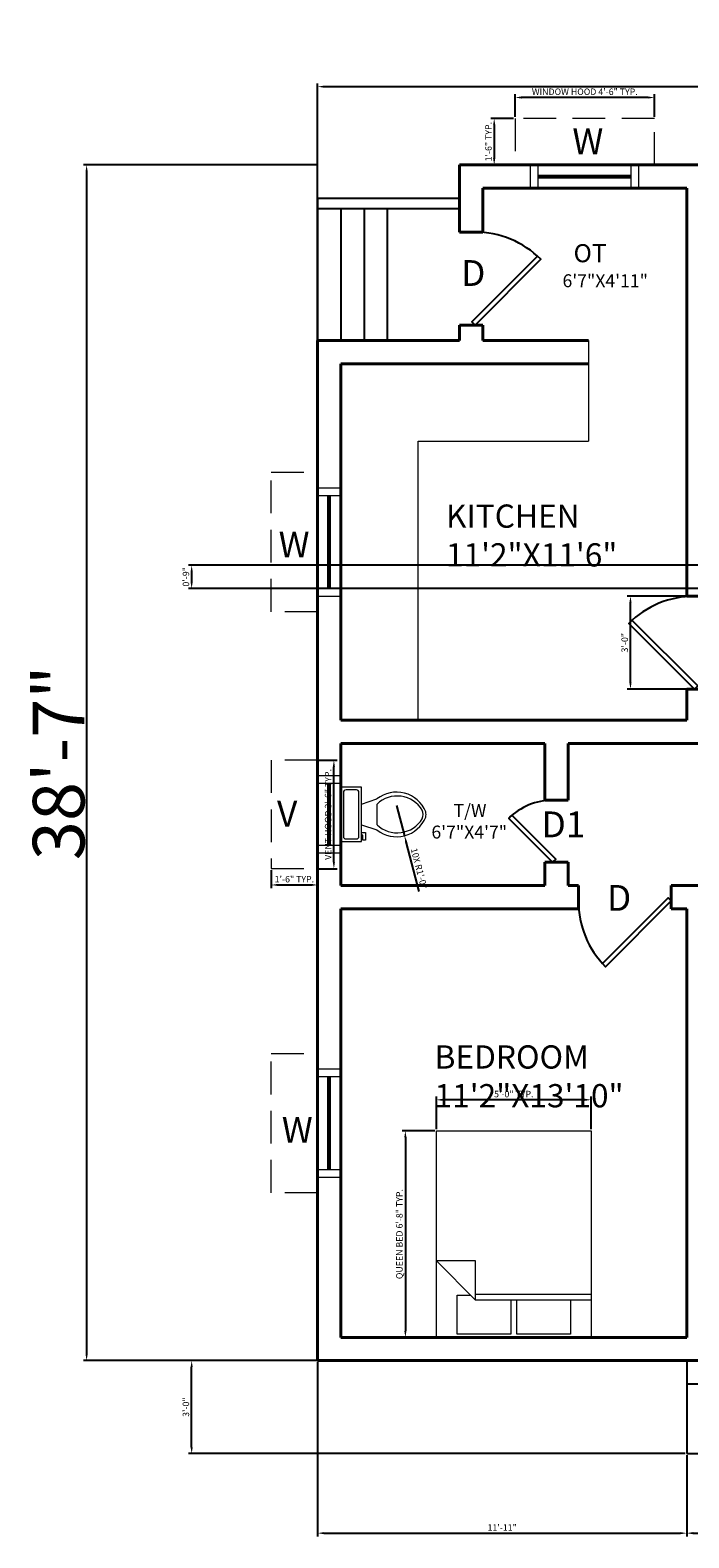
# Model space of a CAD drawing. Units: inches. Extents: x 4878 to 9282, y 5367 to 6617.
# Tile 4 of 14: x 4878 to 5133, y 5787 to 6371. Entities that reach past the tile are written whole.
import ezdxf

# ---------------------------------------------------------------- set-up
doc = ezdxf.new("R2010")
doc.units = ezdxf.units.IN
doc.linetypes.add('DASHED', pattern=[19.05, 12.7, -6.35])
for name, color, linetype, lineweight in [('A-ANNO-DIMS', 2, 'Continuous', 18), ('A-ANNO-TEXT', 7, 'Continuous', 18), ('A-AREA-IDEN', 4, 'Continuous', 18), ('A-DOOR', 3, 'Continuous', 25), ('A-FLOR-FIXT', 9, 'Continuous', 20), ('A-FLOR-STRS', 7, 'Continuous', 25), ('A-FURN', 8, 'Continuous', 18), ('A-GLAZ', 30, 'Continuous', 20), ('A-ROOF-OVHD', 8, 'DASHED', 13), ('A-WALL', 7, 'Continuous', 40)]:
    doc.layers.add(name, color=color, linetype=linetype, lineweight=lineweight)
doc.styles.get("Standard").update_dxf_attribs({"font": 'arial.ttf'})
doc.dimstyles.new('ISO-25', dxfattribs={"dimtxt": 2.5, "dimasz": 2.5, "dimexe": 1.25, "dimexo": 0.625, "dimtad": 1, "dimdec": 0, "dimlunit": 3, "dimtxsty": 'Standard', "dimcen": 2.5, "dimadec": 0, "dimazin": 0, "dimtfac": 1, "dimtdec": 0, "dimtmove": 0, "dimatfit": 3, "dimfxl": 1, "dimarcsym": 0})

# ---------------------------------------------------------------- blocks, each defined once
blk = doc.blocks.new('Bed - Queen')
for p, q in [((0, -80.00003), (0, 0)), ((0, 0), (59.99999, 0)), ((59.99999, 0), (59.99999, -80.00003)), ((7.99999, -1.2), (28.79998, -1.2)), ((7.99999, -14.4), (7.99999, -1.2)), ((28.79998, -1.2), (28.79998, -14.4)), ((31.19999, -1.2), (51.99999, -1.2)), ((31.19999, -14.4), (31.19999, -1.2)), ((51.99999, -1.2), (51.99999, -16.4)), ((0, -14.4), (44.8, -14.4)), ((44.8, -16.8), (0, -16.8)), ((59.99999, -29.6), (44.8, -14.4)), ((44.8, -14.4), (44.8, -29.6)), ((51.99999, -16.4), (46.79936, -16.4)), ((44.8, -29.6), (59.99999, -29.6)), ((59.99999, -80.00003), (0, -80.00003))]:
    blk.add_line(p, q)
blk = doc.blocks.new('Toilet - top')
for p, q in [((9.5, -6), (9.5, -2)), ((-10, -8.5), (-8, -8.5)), ((-10, -9.5), (-10, -8.5)), ((-7, -9.5), (-10, -9.5)), ((-8, -8.5), (-8, -8)), ((-7, -8), (-7, -9.5)), ((-4, -8), (-6, -14)), ((4, -8), (6, -14)), ((4, -14), (-4, -14))]:
    blk.add_line(p, q)
blk.add_lwpolyline([(10.5, -8), (10.5, 0), (-10.5, 0), (-10.5, -8)], close=True)
for points in [[(-9.5, -2), (-9.5, -6)], [(8.5, -1), (-8.5, -1)], [(-8.5, -7), (8.5, -7)]]:
    blk.add_lwpolyline(points)
for centre, radius, start, end in [((-8.62, -1.88), 0.884, 81.8699, 188.1301), ((8.62, -1.88), 0.884, 351.8699, 98.1301), ((-8.62, -6.12), 0.884, 171.8699, 278.1301), ((8.62, -6.12), 0.884, 261.8699, 8.1301), ((3.52, -21.58), 12.17, 141.46911, 247.97143), ((4.2, -21.82), 11.33, 136.36773, 238.94682), ((-3.52, -21.58), 12.17, 292.02843, 38.53071), ((-4.2, -21.82), 11.33, 301.05301, 43.63209), ((0, -27.88), 4, 245.73182, 294.26817), ((0, -29), 4, 254.86053, 285.13947)]:
    blk.add_arc(centre, radius, start, end)
blk = doc.blocks.new('*U11')
for p, q in [((-36, 0), (-36, 6)), ((0, 0), (0, 6))]:
    blk.add_line(p, q)
blk.add_lwpolyline([(0, 0), (-25.46, -25.46), (-26.69, -24.22), (-1.24, 1.24)], close=True)
blk.add_arc((0, 0), 36, 180, 225)
blk = doc.blocks.new('*U12')
for p, q in [((-24, 0), (-24, 6)), ((0, 0), (0, 6))]:
    blk.add_line(p, q)
blk.add_lwpolyline([(0, 0), (-16.97, -16.97), (-18.21, -15.73), (-1.24, 1.24)], close=True)
blk.add_arc((0, 0), 24, 180, 225)
blk = doc.blocks.new('*U8')
for p, q in [((-36, 0), (-36, 6)), ((0, 0), (0, 6))]:
    blk.add_line(p, q)
blk.add_lwpolyline([(0, 0), (-25.46, -25.46), (-26.69, -24.22), (-1.24, 1.24)], close=True)
blk.add_arc((0, 0), 36, 180, 225)
blk = doc.blocks.new('*U13')
for p, q in [((0, 0), (0, -6)), ((-36, 0), (-36, -6))]:
    blk.add_line(p, q)
blk.add_lwpolyline([(0, 0), (-25.46, 25.46), (-26.69, 24.22), (-1.24, -1.24)], close=True)
blk.add_arc((0, 0), 36, 135, 180)
blk = doc.blocks.new('*D16')
at = {"layer": 'A-ANNO-DIMS', "color": 0, "lineweight": -2, "transparency": 16777216}
for p, q in [((4988.98, 6183.27), (4988.98, 6350.19)), ((5442.98, 6348.94), (4991.48, 6348.94)), ((5445.48, 6183.27), (5445.48, 6350.19))]:
    blk.add_line(p, q, dxfattribs=at)
at = {"layer": 'A-ANNO-DIMS', "color": 0, "transparency": 16777216}
for points in [[(4991.48, 6349.36), (4991.48, 6348.53), (4988.98, 6348.94)], [(5442.98, 6349.36), (5442.98, 6348.53), (5445.48, 6348.94)]]:
    blk.add_solid(points, dxfattribs=at)
at = {"layer": 'Defpoints', "color": 0, "transparency": 16777216}
for p in [(4988.98, 6348.94), (4988.98, 6182.64), (5445.48, 6182.64)]:
    blk.add_point(p, dxfattribs=at)
at = {"layer": 'A-ANNO-DIMS', "color": 0, "transparency": 16777216, "insert": (5217.23, 6359.79), "char_height": 2.5, "attachment_point": 5}
blk.add_mtext('{\\H8x;38\'-1"}', dxfattribs=at)
blk = doc.blocks.new('*D17')
at = {"layer": 'A-ANNO-DIMS', "color": 0, "lineweight": -2, "transparency": 16777216}
for p, q in [((4988.98, 6318.64), (4898.23, 6318.64)), ((4899.48, 6316.14), (4899.48, 5858.14)), ((4988.98, 5855.64), (4898.23, 5855.64))]:
    blk.add_line(p, q, dxfattribs=at)
at = {"layer": 'A-ANNO-DIMS', "color": 0, "transparency": 16777216}
for points in [[(4899.07, 6316.14), (4899.9, 6316.14), (4899.48, 6318.64)], [(4899.07, 5858.14), (4899.9, 5858.14), (4899.48, 5855.64)]]:
    blk.add_solid(points, dxfattribs=at)
at = {"layer": 'Defpoints', "color": 0, "transparency": 16777216}
for p in [(4989.6, 6318.64), (4899.48, 5855.64), (4989.6, 5855.64)]:
    blk.add_point(p, dxfattribs=at)
at = {"layer": 'A-ANNO-DIMS', "color": 0, "transparency": 16777216, "insert": (4888.64, 6087.14), "char_height": 2.5, "attachment_point": 5, "rotation": 90}
blk.add_mtext('{\\H8x;38\'-7"}', dxfattribs=at)
blk = doc.blocks.new('WINDOW-PLAN-36IN')
for p, q in [((0, 0), (0, 9)), ((3, 0), (3, 9)), ((39, 0), (39, 9)), ((42, 0), (42, 9)), ((3, 5), (39, 5)), ((3, 4.5), (39, 4.5)), ((3, 4), (39, 4))]:
    blk.add_line(p, q)
blk = doc.blocks.new('WINDOW-PLAN-24IN')
for p, q in [((9, 30), (0, 30)), ((9, 27), (0, 27)), ((4, 3), (4, 27)), ((4.5, 3), (4.5, 27)), ((5, 3), (5, 27)), ((9, 3), (0, 3)), ((9, 0), (0, 0))]:
    blk.add_line(p, q)
blk = doc.blocks.new('WINDOW-HOOD-54IN')
for p, q in [((0, 18), (0, 0)), ((54, 0), (54, 18)), ((0, 0), (54, 0))]:
    blk.add_line(p, q)
blk = doc.blocks.new('WINDOW-HOOD-42IN')
for p, q in [((18, 42), (0, 42)), ((0, 42), (0, 0)), ((0, 0), (18, 0))]:
    blk.add_line(p, q)
blk = doc.blocks.new('*D43')
at = {"layer": 'A-ANNO-DIMS', "color": 0, "lineweight": -2, "transparency": 16777216}
for p, q in [((5065.48, 6337.27), (5065.48, 6345.99)), ((5119.48, 6337.27), (5119.48, 6345.99)), ((5116.98, 6344.74), (5067.98, 6344.74))]:
    blk.add_line(p, q, dxfattribs=at)
at = {"layer": 'A-ANNO-DIMS', "color": 0, "transparency": 16777216}
for points in [[(5067.98, 6345.16), (5067.98, 6344.33), (5065.48, 6344.74)], [(5116.98, 6345.16), (5116.98, 6344.33), (5119.48, 6344.74)]]:
    blk.add_solid(points, dxfattribs=at)
at = {"layer": 'Defpoints', "color": 0, "transparency": 16777216}
for p in [(5065.48, 6344.74), (5065.48, 6336.64), (5119.48, 6336.64)]:
    blk.add_point(p, dxfattribs=at)
at = {"layer": 'A-ANNO-DIMS', "color": 0, "transparency": 16777216, "insert": (5092.48, 6346.66), "char_height": 2.5, "attachment_point": 5}
blk.add_mtext('WINDOW HOOD 4\'-6" TYP.', dxfattribs=at)
blk = doc.blocks.new('*D44')
at = {"layer": 'A-ANNO-DIMS', "color": 0, "lineweight": -2, "transparency": 16777216}
for p, q in [((5064.85, 6336.64), (5056.13, 6336.64)), ((5057.38, 6334.14), (5057.38, 6321.14)), ((5064.85, 6318.64), (5056.13, 6318.64))]:
    blk.add_line(p, q, dxfattribs=at)
at = {"layer": 'A-ANNO-DIMS', "color": 0, "transparency": 16777216}
for points in [[(5056.96, 6334.14), (5057.79, 6334.14), (5057.38, 6336.64)], [(5056.96, 6321.14), (5057.79, 6321.14), (5057.38, 6318.64)]]:
    blk.add_solid(points, dxfattribs=at)
at = {"layer": 'Defpoints', "color": 0, "transparency": 16777216}
for p in [(5065.48, 6336.64), (5057.38, 6318.64), (5065.48, 6318.64)]:
    blk.add_point(p, dxfattribs=at)
at = {"layer": 'A-ANNO-DIMS', "color": 0, "transparency": 16777216, "insert": (5055.48, 6327.64), "char_height": 2.5, "attachment_point": 5, "rotation": 90}
blk.add_mtext('1\'-6" TYP.', dxfattribs=at)
blk = doc.blocks.new('*D45')
at = {"layer": 'A-ANNO-DIMS', "color": 0, "lineweight": -2, "transparency": 16777216}
for p, q in [((4989.6, 6088.14), (4996.53, 6088.14)), ((4995.28, 6048.64), (4995.28, 6085.64)), ((4989.6, 6046.14), (4996.53, 6046.14))]:
    blk.add_line(p, q, dxfattribs=at)
at = {"layer": 'A-ANNO-DIMS', "color": 0, "transparency": 16777216}
for points in [[(4994.86, 6085.64), (4995.69, 6085.64), (4995.28, 6088.14)], [(4994.86, 6048.64), (4995.69, 6048.64), (4995.28, 6046.14)]]:
    blk.add_solid(points, dxfattribs=at)
at = {"layer": 'Defpoints', "color": 0, "transparency": 16777216}
for p in [(4988.98, 6088.14), (4995.28, 6088.14), (4988.98, 6046.14)]:
    blk.add_point(p, dxfattribs=at)
at = {"layer": 'A-ANNO-DIMS', "color": 0, "transparency": 16777216, "insert": (4993.36, 6067.14), "char_height": 2.5, "attachment_point": 5, "rotation": 90}
blk.add_mtext('VENT HOOD 3\'-6" TYP.', dxfattribs=at)
blk = doc.blocks.new('*D46')
at = {"layer": 'A-ANNO-DIMS', "color": 0, "lineweight": -2, "transparency": 16777216}
for p, q in [((4970.98, 6045.52), (4970.98, 6038.59)), ((4988.98, 6045.52), (4988.98, 6038.59)), ((4973.48, 6039.84), (4986.48, 6039.84))]:
    blk.add_line(p, q, dxfattribs=at)
at = {"layer": 'A-ANNO-DIMS', "color": 0, "transparency": 16777216}
for points in [[(4973.48, 6040.26), (4973.48, 6039.43), (4970.98, 6039.84)], [(4986.48, 6040.26), (4986.48, 6039.43), (4988.98, 6039.84)]]:
    blk.add_solid(points, dxfattribs=at)
at = {"layer": 'Defpoints', "color": 0, "transparency": 16777216}
for p in [(4970.98, 6046.14), (4988.98, 6046.14), (4988.98, 6039.84)]:
    blk.add_point(p, dxfattribs=at)
at = {"layer": 'A-ANNO-DIMS', "color": 0, "transparency": 16777216, "insert": (4979.98, 6041.75), "char_height": 2.5, "attachment_point": 5}
blk.add_mtext('1\'-6" TYP.', dxfattribs=at)
blk = doc.blocks.new('*D53')
at = {"layer": 'A-ANNO-DIMS', "color": 0, "lineweight": -2, "transparency": 16777216}
for p, q in [((5034.35, 5944.64), (5021.73, 5944.64)), ((5022.98, 5942.14), (5022.98, 5867.14)), ((5034.35, 5864.64), (5021.73, 5864.64))]:
    blk.add_line(p, q, dxfattribs=at)
at = {"layer": 'A-ANNO-DIMS', "color": 0, "transparency": 16777216}
for points in [[(5022.56, 5942.14), (5023.39, 5942.14), (5022.98, 5944.64)], [(5022.56, 5867.14), (5023.39, 5867.14), (5022.98, 5864.64)]]:
    blk.add_solid(points, dxfattribs=at)
at = {"layer": 'Defpoints', "color": 0, "transparency": 16777216}
for p in [(5034.98, 5944.64), (5022.98, 5864.64), (5034.98, 5864.64)]:
    blk.add_point(p, dxfattribs=at)
at = {"layer": 'A-ANNO-DIMS', "color": 0, "transparency": 16777216, "insert": (5020.98, 5904.64), "char_height": 2.5, "attachment_point": 5, "rotation": 90}
blk.add_mtext('QUEEN BED 6\'-8" TYP.', dxfattribs=at)
blk = doc.blocks.new('*D54')
at = {"layer": 'A-ANNO-DIMS', "color": 0, "lineweight": -2, "transparency": 16777216}
for p, q in [((5034.98, 5945.27), (5034.98, 5957.89)), ((5092.48, 5956.64), (5037.48, 5956.64)), ((5094.98, 5945.27), (5094.98, 5957.89))]:
    blk.add_line(p, q, dxfattribs=at)
at = {"layer": 'A-ANNO-DIMS', "color": 0, "transparency": 16777216}
for points in [[(5037.48, 5957.06), (5037.48, 5956.23), (5034.98, 5956.64)], [(5092.48, 5957.06), (5092.48, 5956.23), (5094.98, 5956.64)]]:
    blk.add_solid(points, dxfattribs=at)
at = {"layer": 'Defpoints', "color": 0, "transparency": 16777216}
for p in [(5034.98, 5956.64), (5034.98, 5944.64), (5094.98, 5944.64)]:
    blk.add_point(p, dxfattribs=at)
at = {"layer": 'A-ANNO-DIMS', "color": 0, "transparency": 16777216, "insert": (5064.98, 5958.55), "char_height": 2.5, "attachment_point": 5}
blk.add_mtext('5\'-0" TYP.', dxfattribs=at)
blk = doc.blocks.new('*D100')
at = {"layer": 'A-ANNO-DIMS', "color": 0, "lineweight": -2, "transparency": 16777216}
for p, q in [((4988.35, 5855.64), (4938.93, 5855.64)), ((4940.18, 5822.14), (4940.18, 5853.14)), ((5131.35, 5819.64), (4938.93, 5819.64))]:
    blk.add_line(p, q, dxfattribs=at)
at = {"layer": 'A-ANNO-DIMS', "color": 0, "transparency": 16777216}
for points in [[(4939.76, 5853.14), (4940.59, 5853.14), (4940.18, 5855.64)], [(4939.76, 5822.14), (4940.59, 5822.14), (4940.18, 5819.64)]]:
    blk.add_solid(points, dxfattribs=at)
at = {"layer": 'Defpoints', "color": 0, "transparency": 16777216}
for p in [(4940.18, 5855.64), (4988.98, 5855.64), (5131.98, 5819.64)]:
    blk.add_point(p, dxfattribs=at)
at = {"layer": 'A-ANNO-DIMS', "color": 0, "transparency": 16777216, "insert": (4938.27, 5837.64), "char_height": 2.5, "attachment_point": 5, "rotation": 90}
blk.add_mtext('3\'-0"', dxfattribs=at)
blk = doc.blocks.new('*D101')
at = {"layer": 'A-ANNO-DIMS', "color": 0, "lineweight": -2, "transparency": 16777216}
for p, q in [((4988.98, 5855.02), (4988.98, 5787.59)), ((5131.98, 5819.02), (5131.98, 5787.59)), ((4991.48, 5788.84), (5129.48, 5788.84))]:
    blk.add_line(p, q, dxfattribs=at)
at = {"layer": 'A-ANNO-DIMS', "color": 0, "transparency": 16777216}
for points in [[(4991.48, 5789.26), (4991.48, 5788.43), (4988.98, 5788.84)], [(5129.48, 5789.26), (5129.48, 5788.43), (5131.98, 5788.84)]]:
    blk.add_solid(points, dxfattribs=at)
at = {"layer": 'Defpoints', "color": 0, "transparency": 16777216}
for p in [(4988.98, 5855.64), (5131.98, 5819.64), (5131.98, 5788.84)]:
    blk.add_point(p, dxfattribs=at)
at = {"layer": 'A-ANNO-DIMS', "color": 0, "transparency": 16777216, "insert": (5060.48, 5790.72), "char_height": 2.5, "attachment_point": 5}
blk.add_mtext('11\'-11"', dxfattribs=at)
blk = doc.blocks.new('*D102')
at = {"layer": 'A-ANNO-DIMS', "color": 0, "lineweight": -2, "transparency": 16777216}
for p, q in [((5131.98, 5819.02), (5131.98, 5787.59)), ((5311.48, 5819.02), (5311.48, 5787.59)), ((5134.48, 5788.84), (5308.98, 5788.84))]:
    blk.add_line(p, q, dxfattribs=at)
at = {"layer": 'A-ANNO-DIMS', "color": 0, "transparency": 16777216}
for points in [[(5134.48, 5789.26), (5134.48, 5788.43), (5131.98, 5788.84)], [(5308.98, 5789.26), (5308.98, 5788.43), (5311.48, 5788.84)]]:
    blk.add_solid(points, dxfattribs=at)
at = {"layer": 'Defpoints', "color": 0, "transparency": 16777216}
for p in [(5131.98, 5819.64), (5311.48, 5819.64), (5311.48, 5788.84)]:
    blk.add_point(p, dxfattribs=at)
at = {"layer": 'A-ANNO-DIMS', "color": 0, "transparency": 16777216, "insert": (5221.73, 5790.76), "char_height": 2.5, "attachment_point": 5}
blk.add_mtext('14\'-11 1/2"', dxfattribs=at)
blk = doc.blocks.new('*D105')
at = {"layer": 'A-ANNO-DIMS', "color": 0, "lineweight": -2, "transparency": 16777216}
for p, q in [((5140.35, 6151.64), (5108.93, 6151.64)), ((5110.18, 6118.14), (5110.18, 6149.14)), ((5140.35, 6115.64), (5108.93, 6115.64))]:
    blk.add_line(p, q, dxfattribs=at)
at = {"layer": 'A-ANNO-DIMS', "color": 0, "transparency": 16777216}
for points in [[(5109.76, 6149.14), (5110.59, 6149.14), (5110.18, 6151.64)], [(5109.76, 6118.14), (5110.59, 6118.14), (5110.18, 6115.64)]]:
    blk.add_solid(points, dxfattribs=at)
at = {"layer": 'Defpoints', "color": 0, "transparency": 16777216}
for p in [(5110.18, 6151.64), (5140.98, 6151.64), (5140.98, 6115.64)]:
    blk.add_point(p, dxfattribs=at)
at = {"layer": 'A-ANNO-DIMS', "color": 0, "transparency": 16777216, "insert": (5108.27, 6133.64), "char_height": 2.5, "attachment_point": 5, "rotation": 90}
blk.add_mtext('3\'-0"', dxfattribs=at)
blk = doc.blocks.new('*D114')
at = {"layer": 'A-ANNO-DIMS', "color": 0, "lineweight": -2, "transparency": 16777216}
for p, q in [((5140.35, 6163.64), (4938.93, 6163.64)), ((4940.18, 6161.14), (4940.18, 6157.14)), ((5140.35, 6154.64), (4938.93, 6154.64))]:
    blk.add_line(p, q, dxfattribs=at)
at = {"layer": 'A-ANNO-DIMS', "color": 0, "transparency": 16777216}
for points in [[(4939.76, 6161.14), (4940.59, 6161.14), (4940.18, 6163.64)], [(4939.76, 6157.14), (4940.59, 6157.14), (4940.18, 6154.64)]]:
    blk.add_solid(points, dxfattribs=at)
at = {"layer": 'Defpoints', "color": 0, "transparency": 16777216}
for p in [(5140.98, 6163.64), (4940.18, 6154.64), (5140.98, 6154.64)]:
    blk.add_point(p, dxfattribs=at)
at = {"layer": 'A-ANNO-DIMS', "color": 0, "transparency": 16777216, "insert": (4938.28, 6159.14), "char_height": 2.5, "attachment_point": 5, "rotation": 90}
blk.add_mtext('0\'-9"', dxfattribs=at)
blk = doc.blocks.new('*D126')
at = {"layer": 'A-ANNO-DIMS', "color": 0, "lineweight": -2, "transparency": 16777216}
for p, q in [((5019.56, 6070.66), (5022.65, 6058.89)), ((5028.33, 6037.26), (5023.29, 6056.48))]:
    blk.add_line(p, q, dxfattribs=at)
at = {"layer": 'A-ANNO-DIMS', "color": 0, "transparency": 16777216}
blk.add_solid([(5023.69, 6056.58), (5022.88, 6056.37), (5022.65, 6058.89)], dxfattribs=at)
at = {"layer": 'Defpoints', "color": 0, "transparency": 16777216}
for p in [(5019.56, 6070.66), (5022.65, 6058.89)]:
    blk.add_point(p, dxfattribs=at)
at = {"layer": 'A-ANNO-DIMS', "color": 0, "transparency": 16777216, "insert": (5027.97, 6046.14), "char_height": 2.5, "attachment_point": 5, "rotation": 284.72178}
blk.add_mtext('10X R1\'-0"', dxfattribs=at)

msp = doc.modelspace()

# ---------------------------------------------------------------- linework, layer by layer
at = {"layer": 'A-FLOR-FIXT'}
for p, q in [((5093.98, 6250.64), (5093.98, 6211.64)), ((5027.98, 6103.64), (5027.98, 6211.64)), ((5027.98, 6211.64), (5093.98, 6211.64))]:
    msp.add_line(p, q, dxfattribs=at)
at = {"layer": 'A-FLOR-STRS'}
for p, q in [((5043.98, 6305.64), (4988.98, 6305.64)), ((4988.98, 6305.64), (4988.98, 6250.64)), ((5043.98, 6301.64), (4988.98, 6301.64)), ((4997.98, 6301.64), (4997.98, 6250.64)), ((5006.98, 6301.64), (5006.98, 6250.64)), ((5015.98, 6301.64), (5015.98, 6250.64)), ((5131.98, 5855.64), (5131.98, 5819.64)), ((5131.98, 5846.64), (5311.48, 5846.64)), ((5131.98, 5819.64), (5311.48, 5819.64))]:
    msp.add_line(p, q, dxfattribs=at)
at = {"layer": 'A-WALL'}
for p, q in [((5043.98, 6318.64), (5140.98, 6318.64)), ((5043.98, 6318.64), (5043.98, 6292.64)), ((5052.98, 6309.64), (5131.98, 6309.64)), ((5052.98, 6309.64), (5052.98, 6292.64)), ((5131.98, 6309.64), (5131.98, 6151.64)), ((5043.98, 6292.64), (5052.98, 6292.64)), ((5043.98, 6256.64), (5052.98, 6256.64)), ((5043.98, 6256.64), (5043.98, 6250.64)), ((5052.98, 6256.64), (5052.98, 6250.64)), ((4988.98, 6250.64), (5043.98, 6250.64)), ((4988.98, 5855.64), (4988.98, 6250.64)), ((5052.98, 6250.64), (5093.98, 6250.64)), ((4997.98, 6241.64), (5093.98, 6241.64)), ((4997.98, 6103.64), (4997.98, 6241.64)), ((5131.98, 6151.64), (5140.98, 6151.64)), ((5131.98, 6115.64), (5140.98, 6115.64)), ((5131.98, 6115.64), (5131.98, 6103.64)), ((5131.98, 6103.64), (4997.98, 6103.64)), ((4997.98, 6039.64), (4997.98, 6094.64)), ((5076.98, 6094.64), (4997.98, 6094.64)), ((5076.98, 6072.64), (5076.98, 6094.64)), ((5140.98, 6094.64), (5085.98, 6094.64)), ((5085.98, 6072.64), (5085.98, 6094.64)), ((5085.98, 6072.64), (5076.98, 6072.64)), ((5076.98, 6039.64), (5076.98, 6048.64)), ((5085.98, 6048.64), (5076.98, 6048.64)), ((5085.98, 6039.64), (5085.98, 6048.64)), ((5076.98, 6039.64), (4997.98, 6039.64)), ((5089.98, 6039.64), (5085.98, 6039.64)), ((5089.98, 6030.64), (5089.98, 6039.64)), ((5125.98, 6030.64), (5125.98, 6039.64)), ((5140.98, 6039.64), (5125.98, 6039.64)), ((4997.98, 5864.64), (4997.98, 6030.64)), ((5089.98, 6030.64), (4997.98, 6030.64)), ((5131.98, 6030.64), (5125.98, 6030.64)), ((5131.98, 5864.64), (5131.98, 6030.64)), ((5131.98, 5864.64), (4997.98, 5864.64)), ((5140.98, 5855.64), (4988.98, 5855.64))]:
    msp.add_line(p, q, dxfattribs=at)

# ---------------------------------------------------------------- block references
at = {"layer": 'A-DOOR', "rotation": 270}
for name, p in [('*U13', (5049.98, 6256.64)), ('*U8', (5134.98, 6115.64)), ('*U12', (5079.98, 6048.64))]:
    msp.add_blockref(name, p, dxfattribs=at)
at = {"layer": 'A-DOOR'}
msp.add_blockref('*U11', (5125.98, 6033.64), dxfattribs=at)
at = {"layer": 'A-FLOR-FIXT', "rotation": 89.99999999999999}
msp.add_blockref('Toilet - top', (4997.98, 6067.14), dxfattribs=at)
at = {"layer": 'A-FURN', "rotation": 180}
msp.add_blockref('Bed - Queen', (5094.98, 5864.64), dxfattribs=at)
at = {"layer": 'A-GLAZ'}
for name, p in [('WINDOW-PLAN-36IN', (5071.48, 6309.65)), ('WINDOW-PLAN-24IN', (4988.98, 6052.15))]:
    msp.add_blockref(name, p, dxfattribs=at)
at = {"layer": 'A-GLAZ', "extrusion": (0, 0, -1), "zscale": -1, "rotation": 90}
for p in [(-4988.98, 6151.64), (-4988.98, 5926.64)]:
    msp.add_blockref('WINDOW-PLAN-36IN', p, dxfattribs=at)
at = {"layer": 'A-ROOF-OVHD', "rotation": 180}
msp.add_blockref('WINDOW-HOOD-54IN', (5119.48, 6336.64), dxfattribs=at)
at = {"layer": 'A-ROOF-OVHD', "extrusion": (0, 0, -1), "zscale": -1, "rotation": 90}
for p in [(-4970.98, 6145.64), (-4970.98, 5920.64)]:
    msp.add_blockref('WINDOW-HOOD-54IN', p, dxfattribs=at)
at = {"layer": 'A-ROOF-OVHD'}
msp.add_blockref('WINDOW-HOOD-42IN', (4970.98, 6046.15), dxfattribs=at)

# ---------------------------------------------------------------- texts
at = {"layer": 'A-ANNO-TEXT', "char_height": 10, "width": 649.8744, "attachment_point": 1}
for s, insert in [('W', (5087.67, 6332.77)), ('D', (5044.58, 6281.78)), ('W', (4973.87, 6176.68)), ('V', (4973.25, 6072.43)), ('D1', (5075.75, 6068.29)), ('D', (5101.09, 6039.82)), ('W', (4975.1, 5950))]:
    msp.add_mtext(s, dxfattribs=dict(at, insert=insert))
at = {"layer": 'A-AREA-IDEN', "attachment_point": 1}
for s, width, insert, char_height in [('  OT{\\H0.71429x;\\P6\'7"X4\'11"}', 337.032, (5083.86, 6287.96), 7), ('KITCHEN\\P11\'2"X11\'6"', 597.3901, (5038.71, 6187.15), 9), ('    {\\H0.71429x;T/W\\P6\'7"X4\'7"}', 337.032, (5033.07, 6071.15), 7), ('BEDROOM\\P11\'2"X13\'10"', 351.5597, (5034.3, 5977.73), 9)]:
    msp.add_mtext_dynamic_manual_height_columns(s, width=width, gutter_width=12.5, heights=[0], dxfattribs=dict(at, insert=insert, char_height=char_height))

# ---------------------------------------------------------------- dimensions: what is measured, and where the dimension line sits
at = {"layer": 'A-ANNO-DIMS'}
for base, p1, p2, text, override, picture, middle in [((4988.97709281, 6348.94354297), (5445.47709281, 6182.64478635), (4988.97709281, 6182.64478635), '{\\H8x;<>}', {"dimclrd": 0, "dimclre": 0, "dimclrt": 0}, '*D16', (5217.22709281, 6359.786824)), ((4988.98, 6039.84), (4970.98, 6046.14), (4988.98, 6046.14), '<> TYP.', {"dimdec": 1, "dimlfac": 1, "dimrnd": 0, "dimzin": 1, "dimdsep": 46, "dimlunit": 4, "dimfrac": 2}, '*D46', (4979.98, 6041.75))]:
    dim = msp.add_linear_dim(base=base, p1=p1, p2=p2, text=text, dimstyle='ISO-25', override=override, dxfattribs=at)
    dim.commit()
    dim.dimension.update_dxf_attribs({"geometry": picture, "text_midpoint": middle})
for base, p1, p2, angle, text, override, picture, middle in [((5065.48, 6344.74), (5119.48, 6336.64), (5065.48, 6336.64), 180, 'WINDOW HOOD <> TYP.', {"dimdec": 1, "dimlfac": 1, "dimrnd": 0, "dimzin": 1, "dimdsep": 46, "dimlunit": 4, "dimfrac": 2}, '*D43', (5092.48, 6346.66)), ((5057.38, 6318.64), (5065.48, 6336.64), (5065.48, 6318.64), 270, '<> TYP.', {"dimdec": 1, "dimlfac": 1, "dimrnd": 0, "dimzin": 1, "dimdsep": 46, "dimlunit": 4, "dimfrac": 2}, '*D44', (5055.48, 6327.64)), ((4899.48, 5855.64), (4989.6, 6318.64), (4989.6, 5855.64), 90, '{\\H8x;<>}', {"dimclrd": 0, "dimclre": 0, "dimclrt": 0}, '*D17', (4888.64, 6087.14)), ((4995.28, 6088.14), (4988.98, 6046.14), (4988.98, 6088.14), 90, 'VENT HOOD <> TYP.', {"dimdec": 1, "dimlfac": 1, "dimrnd": 0, "dimzin": 1, "dimdsep": 46, "dimlunit": 4, "dimfrac": 2}, '*D45', (4993.36, 6067.14)), ((5034.98, 5956.64), (5094.98, 5944.64), (5034.98, 5944.64), 180, '<> TYP.', {"dimdec": 1, "dimlfac": 1, "dimrnd": 0, "dimzin": 1, "dimdsep": 46, "dimlunit": 4, "dimfrac": 2}, '*D54', (5064.98, 5958.55)), ((5022.98, 5864.64), (5034.98, 5944.64), (5034.98, 5864.64), 270, 'QUEEN BED <> TYP.', {"dimdec": 1, "dimlfac": 1, "dimrnd": 0, "dimzin": 1, "dimdsep": 46, "dimlunit": 4, "dimfrac": 2}, '*D53', (5020.98, 5904.64))]:
    dim = msp.add_linear_dim(base=base, p1=p1, p2=p2, angle=angle, text=text, dimstyle='ISO-25', override=override, dxfattribs=at)
    dim.commit()
    dim.dimension.update_dxf_attribs({"geometry": picture, "text_midpoint": middle})
for base, p1, p2, picture, middle in [((4940.18, 6154.64), (5140.98, 6163.64), (5140.98, 6154.64), '*D114', (4938.28, 6159.14)), ((5110.18, 6151.64), (5140.98, 6115.64), (5140.98, 6151.64), '*D105', (5108.27, 6133.64)), ((4940.18, 5855.64), (5131.98, 5819.64), (4988.98, 5855.64), '*D100', (4938.27, 5837.64))]:
    dim = msp.add_linear_dim(base=base, p1=p1, p2=p2, angle=90, dimstyle='ISO-25', override={"dimdec": 1, "dimlfac": 1, "dimrnd": 0, "dimzin": 1, "dimdsep": 46, "dimlunit": 4, "dimfrac": 2}, dxfattribs=at)
    dim.commit()
    dim.dimension.update_dxf_attribs({"geometry": picture, "text_midpoint": middle})
dim = msp.add_radius_dim(center=(5019.56, 6070.66), mpoint=(5022.65, 6058.89), text='10X <>', dimstyle='ISO-25', override={"dimdec": 1, "dimlfac": 1, "dimrnd": 0, "dimzin": 1, "dimdsep": 46, "dimlunit": 4, "dimfrac": 2}, dxfattribs=at)
dim.commit()
dim.dimension.update_dxf_attribs({"geometry": '*D126', "text_midpoint": (5027.97, 6046.14)})
for base, p1, p2, picture, middle in [((5131.98, 5788.84), (4988.98, 5855.64), (5131.98, 5819.64), '*D101', (5060.48, 5790.72)), ((5311.48, 5788.84), (5131.98, 5819.64), (5311.48, 5819.64), '*D102', (5221.73, 5790.76))]:
    dim = msp.add_linear_dim(base=base, p1=p1, p2=p2, dimstyle='ISO-25', override={"dimdec": 1, "dimlfac": 1, "dimrnd": 0, "dimzin": 1, "dimdsep": 46, "dimlunit": 4, "dimfrac": 2}, dxfattribs=at)
    dim.commit()
    dim.dimension.update_dxf_attribs({"geometry": picture, "text_midpoint": middle})

doc.saveas('drawing.dxf')
